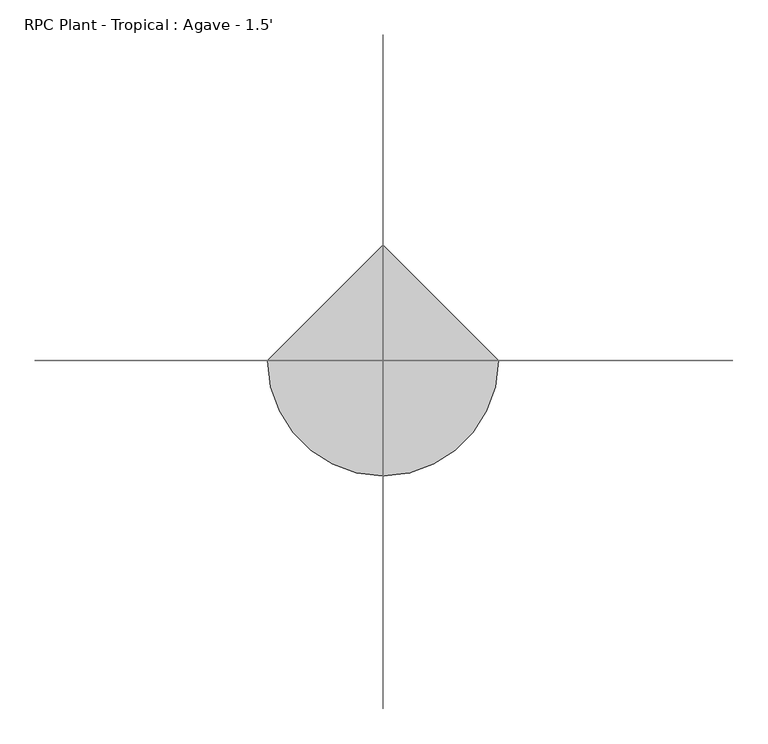
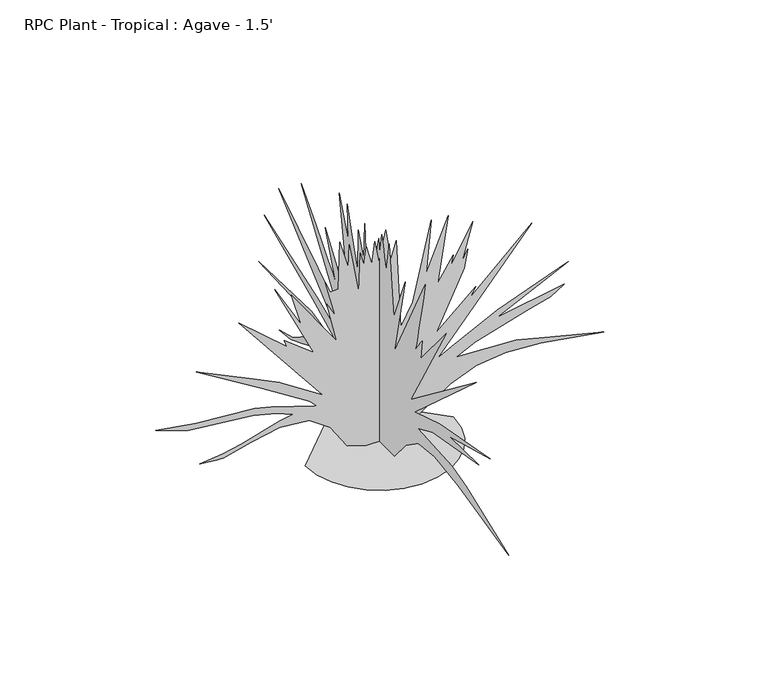
"""IFC4 building model written with IfcOpenShell, lengths in millimetres: geographic element geometry, RPC Plant - Tropical : Agave - 1.5'."""

from ifc_helpers import new_model, si_unit, origin, place, context, project, spatial, triangles, source, transform, mapped, element, save


def rpc_plant_tropical_agave_1_5_74a88192(model_context):
    return source(origin(), model_context, "Body", "Tessellation", [
        triangles([(-200.9449838, 0.0, 1.26e-05), (-195.6326446, -46.0431244, 1.26e-05), (-180.5030448, -88.3267035, 1.26e-05), (-156.767902, -125.6386611, 1.26e-05), (-125.6386611, -156.767902, 1.26e-05), (-88.3267035, -180.5030448, 1.26e-05), (-46.0431244, -195.6326446, 1.26e-05), (8.8e-06, -200.9449838, 1.26e-05), (46.0431244, -195.6326446, 1.26e-05), (88.3267035, -180.5030448, 1.26e-05), (125.6386611, -156.767902, 1.26e-05), (156.767902, -125.6386611, 1.26e-05), (180.5030448, -88.3267035, 1.26e-05), (195.6326446, -46.0431244, 1.26e-05), (200.9449838, 1.76e-05, 1.26e-05), (-2.64e-05, 200.9449838, 1.26e-05), (-33.2531301, 1.5e-06, 3.4e-06), (-87.23451, 2.8e-06, 17.5224236), (-132.8827502, 6e-07, 86.7952563), (-190.7246956, 7e-07, 127.5544962), (-269.7661646, 3.8e-06, 134.8537872), (-346.3140358, 8.1e-06, 118.9056237), (-422.3684778, 1.25e-05, 99.9853214), (-439.494867, 1.32e-05, 100.6714532), (-487.1046427, 1.5e-05, 105.5966886), (-424.417408, 1.19e-05, 112.1471881), (-376.4520218, 9.2e-06, 122.3864432), (-270.8011305, 2.7e-06, 153.1431596), (-234.2809759, 7e-07, 159.7728966), (-277.816618, 1.6e-06, 177.4516504), (-342.3583906, 3.4e-06, 194.3836474), (-519.0443356, 1e-05, 213.4357003), (-606.9487083, 1.2e-05, 243.4998354), (-498.5956201, 8.4e-06, 225.4410903), (-337.7084928, 2.1e-06, 212.3075897), (-293.8098278, 8e-07, 201.4407929), (-170.2543063, -2.2e-06, 161.4147659), (-187.2980515, -2.6e-06, 180.4058487), (-317.7989522, -1.8e-06, 262.7469528), (-496.9530968, -5e-07, 373.1940448), (-341.7894573, -2.9e-06, 298.7310027), (-272.0403172, -3.9e-06, 264.8422827), (-153.8374304, -4.5e-06, 187.6821124), (-382.0332218, -1.15e-05, 473.3378594), (-250.6978699, -1.05e-05, 360.0605441), (-257.2649473, -1.14e-05, 379.7607951), (-178.4629077, -1.11e-05, 317.3766306), (-283.5322938, -1.95e-05, 535.7236954), (-211.2970046, -1.52e-05, 409.312843), (-239.2062203, -1.96e-05, 504.532467), (-116.0780891, -1.45e-05, 328.8686254), (-142.3454357, -2.02e-05, 443.7891543), (-119.3614643, -1.88e-05, 402.7460927), (-147.270671, -2.38e-05, 507.8141344), (-132.9569099, -2.26e-05, 475.9049266), (-111.0309408, -2.35e-05, 475.9320325), (-107.8694877, -3.16e-05, 609.6005087), (-84.5692021, -2.79e-05, 529.295781), (-81.6021412, -3.18e-05, 593.1819251), (-55.3351308, -2.42e-05, 447.0708218), (-52.051415, -3.1e-05, 558.708993), (-42.2012849, -2.92e-05, 520.9476351), (-35.6345346, -3.25e-05, 571.8424936), (-20.8591737, -2.98e-05, 516.023408), (-12.6506665, -3.39e-05, 578.4092803), (-1.1586981, -3.07e-05, 516.023408), (16.9000563, -3.66e-05, 601.3911987), (31.6754171, -3.18e-05, 511.0992173), (46.4508802, -3.54e-05, 560.3481371), (57.9428658, -2.09e-05, 307.5265051), (90.7766266, -2.59e-05, 368.2698177), (140.6642974, -4.11e-05, 586.605001), (126.8944347, -3.17e-05, 438.8615481), (187.3105871, -4.29e-05, 582.6053541), (158.0866805, -3.07e-05, 399.4610461), (200.7712481, -3.65e-05, 465.1319286), (194.2044977, -3.45e-05, 435.5798807), (253.3059411, -4.34e-05, 542.2904457), (223.7552194, -3.58e-05, 437.222404), (240.1720953, -3.84e-05, 468.4136324), (231.2908968, -3.5e-05, 417.3460373), (154.8033053, -2.22e-05, 258.2751872), (261.5145425, -3.25e-05, 353.4937938), (245.0973215, -3.01e-05, 325.5852502), (414.1930684, -4.68e-05, 481.5471331), (158.0866805, -1.79e-05, 184.3983921), (211.2997297, -2.18e-05, 210.7700382), (320.6156407, -2.98e-05, 264.8422827), (512.6943234, -4.25e-05, 337.0772449), (318.9741348, -2.85e-05, 243.4998354), (502.3819078, -3.84e-05, 275.1540261), (465.5654414, -3.54e-05, 253.17588), (400.5481527, -3.15e-05, 234.7595259), (260.6113273, -2.3e-05, 194.7771735), (208.9798495, -1.92e-05, 169.6230221), (371.5074835, -2.59e-05, 161.4147659), (448.5270919, -2.8e-05, 141.4672734), (609.5564707, -3.26e-05, 100.6714532), (438.7667138, -2.68e-05, 128.2728117), (343.242312, -2.3e-05, 134.8036631), (263.2766261, -1.9e-05, 125.4744088), (193.0049343, -1.43e-05, 97.8246248), (115.3421693, -7.8e-06, 45.5100628), (44.0785186, -1.9e-06, 0.0), (1.2e-06, 26.7781575, 1.21e-05), (2.8e-06, 63.7333918, 1.32e-05), (4.9e-06, 91.2118108, 26.7772105), (8.3e-06, 132.92677, 78.8260843), (1.11e-05, 176.9572038, 107.6236088), (1.38e-05, 232.3665034, 113.1289777), (1.53e-05, 278.1119306, 97.1591404), (1.8e-05, 362.9899801, 61.1154965), (1.98e-05, 415.9778432, 40.3792577), (2.21e-05, 471.1026398, 33.361606), (1.97e-05, 407.172494, 51.8140112), (1.79e-05, 333.0020576, 99.7668755), (1.58e-05, 266.4753407, 130.2140541), (1.34e-05, 214.9972874, 128.5806599), (1.56e-05, 251.3697766, 147.1551893), (2.01e-05, 341.4880222, 162.6979724), (3.05e-05, 567.6227294, 172.7346963), (1.96e-05, 318.4244591, 179.4734928), (1.45e-05, 219.9269284, 158.3250926), (1.09e-05, 159.1792192, 128.5806599), (1.46e-05, 213.2609472, 170.2228038), (2.05e-05, 311.7594953, 220.3624396), (3.38e-05, 541.6977493, 320.6603691), (2e-05, 290.5156066, 236.9330851), (1.47e-05, 196.9382153, 197.5322379), (3.42e-05, 472.7451631, 438.8615481), (1.66e-05, 194.9377015, 264.7396727), (3.18e-05, 366.0345981, 517.6659677), (2.91e-05, 331.7090406, 479.3288455), (2.65e-05, 298.6551353, 442.1771161), (2.41e-05, 268.1432804, 407.3994061), (2.2e-05, 241.444474, 376.1810718), (2.02e-05, 219.8300593, 349.7040905), (1.9e-05, 204.5710888, 329.1615581), (1.82e-05, 196.9382153, 315.7351247), (2.51e-05, 254.3981346, 460.2043588), (2.02e-05, 198.5512891, 378.3282154), (1.97e-05, 193.2335359, 371.1213879), (1.92e-05, 186.8002077, 363.6537841), (1.86e-05, 179.4369216, 355.9694421), (1.8e-05, 171.3295677, 348.1157427), (1.74e-05, 162.6641082, 340.1299656), (1.68e-05, 153.6267783, 332.0585469), (1.61e-05, 144.4038584, 323.9437443), (2.62e-05, 187.0880898, 599.7486754), (2.11e-05, 146.0453733, 489.7564067), (2.43e-05, 150.9706087, 589.9002213), (2.15e-05, 131.2703486, 524.232718), (1.72e-05, 100.0777758, 427.3705708), (2.07e-05, 98.4359156, 547.2146364), (1.76e-05, 73.8104293, 478.2654656), (2.05e-05, 68.8851939, 583.333471), (1.81e-05, 63.0127099, 512.2439149), (1.46e-05, 36.0510948, 437.222404), (1.74e-05, 1.5752787, 581.6909477), (1.6e-05, -1.7081751, 540.6478861), (1.74e-05, -11.4000706, 600.60887), (1.66e-05, -15.9711602, 581.5250058), (1.59e-05, -20.3254695, 563.0236279), (1.52e-05, -24.246283, 545.6838796), (1.46e-05, -27.5167911, 530.0916627), (1.41e-05, -29.9202417, 516.8260843), (1.37e-05, -31.2398582, 506.4696307), (1.35e-05, -31.258891, 499.6048608), (1.57e-05, -46.0343177, 594.8244484), (8.8e-06, -67.3764334, 397.821902), (1.04e-05, -123.1944971, 532.4419916), (5.8e-06, -70.6598086, 300.9597548), (7.6e-06, -216.7715614, 581.6909477), (6.8e-06, -207.9360723, 538.6666843), (5.9e-06, -199.3546012, 497.2104939), (5.1e-06, -191.2818018, 458.8869246), (4.4e-06, -183.9716739, 425.264086), (3.9e-06, -177.6789076, 397.9099417), (3.6e-06, -172.6578296, 378.3891855), (3.4e-06, -169.1620946, 368.2698177), (3.4e-06, -168.0119831, 365.6180537), (3.4e-06, -169.5576736, 367.0032163), (3.3e-06, -173.3493753, 371.7547068), (3.3e-06, -178.9387326, 379.1985838), (3.3e-06, -185.8756638, 388.6609423), (3.2e-06, -193.7113955, 399.4711836), (3.2e-06, -201.9962096, 410.9554027), (1.9e-06, -193.7879352, 355.1363171), (8e-07, -315.274179, 501.2473841), (-3e-07, -147.8199925, 210.6657386), (-7.1e-06, -454.8195494, 445.4282985), (-1.9e-06, -165.8787194, 184.3987372), (-6.1e-06, -284.0816244, 222.1577152), (-1.54e-05, -521.71979, 265.9195789), (-8.3e-06, -328.407716, 213.9491138), (-1.45e-05, -468.6201968, 217.2328341), (-6e-06, -252.4355546, 178.0016531), (-3.7e-06, -180.6540894, 146.639396), (-1.13e-05, -343.1847573, 136.7889344), (-1.47e-05, -408.8522607, 118.7301893), (-2.59e-05, -607.4973667, 41.5700099), (-1.37e-05, -370.6743585, 97.1591404), (-8.3e-06, -260.1791771, 113.3443716), (-5.1e-06, -183.4795891, 105.2979877), (-3.7e-06, -125.5777001, 65.1557931), (-3.1e-06, -70.1362304, 9.2e-06), (-1.1e-06, -25.5007055, 1.06e-05)], [[15, 16, 1], [14, 15, 1], [14, 1, 2], [13, 14, 2], [13, 2, 3], [13, 3, 4], [12, 13, 4], [11, 12, 4], [11, 4, 5], [11, 5, 6], [11, 6, 7], [11, 7, 8], [11, 8, 9], [11, 9, 10], [47, 48, 49], [97, 98, 99], [88, 89, 90], [39, 40, 41], [84, 85, 86], [71, 72, 73], [53, 54, 55], [32, 33, 34], [43, 44, 45], [24, 25, 26], [58, 59, 60], [77, 78, 79], [73, 74, 75], [60, 61, 62], [51, 52, 53], [56, 57, 58], [82, 83, 84], [79, 80, 81], [64, 65, 66], [49, 50, 51], [68, 69, 70], [75, 76, 77], [90, 91, 92], [90, 92, 93], [66, 67, 68], [82, 84, 86], [90, 93, 94], [62, 63, 64], [47, 49, 51], [39, 41, 42], [45, 46, 47], [43, 45, 47], [38, 39, 42], [38, 42, 43], [31, 32, 34], [31, 34, 35], [23, 24, 26], [56, 58, 60], [87, 88, 90], [87, 90, 94], [87, 94, 95], [37, 38, 43], [86, 87, 95], [71, 73, 75], [96, 97, 99], [96, 99, 100], [95, 96, 100], [95, 100, 101], [95, 101, 102], [53, 55, 56], [53, 56, 60], [22, 23, 26], [22, 26, 27], [22, 27, 28], [21, 22, 28], [60, 62, 64], [43, 47, 51], [30, 31, 35], [30, 35, 36], [30, 36, 37], [29, 30, 37], [86, 95, 102], [21, 28, 29], [20, 21, 29], [20, 29, 37], [19, 20, 37], [86, 102, 103], [66, 68, 70], [64, 66, 70], [60, 64, 70], [53, 60, 70], [51, 53, 70], [43, 51, 70], [77, 79, 81], [77, 81, 82], [75, 77, 82], [71, 75, 82], [70, 71, 82], [70, 82, 86], [43, 70, 86], [43, 86, 103], [43, 103, 104], [43, 104, 17], [43, 17, 18], [43, 18, 19], [43, 19, 37], [120, 121, 122], [193, 194, 195], [190, 191, 192], [126, 127, 128], [155, 156, 157], [131, 132, 133], [200, 201, 202], [113, 114, 115], [195, 196, 197], [129, 130, 131], [131, 133, 134], [170, 171, 172], [188, 189, 190], [131, 134, 135], [148, 149, 150], [139, 140, 141], [131, 135, 136], [150, 151, 152], [168, 169, 170], [172, 173, 174], [131, 136, 137], [158, 159, 160], [172, 174, 175], [131, 137, 138], [153, 154, 155], [131, 138, 139], [172, 175, 176], [160, 161, 162], [172, 176, 177], [186, 187, 188], [172, 177, 178], [112, 113, 115], [112, 115, 116], [111, 112, 116], [111, 116, 117], [160, 162, 163], [172, 178, 179], [172, 179, 180], [172, 180, 181], [139, 141, 142], [193, 195, 197], [185, 186, 188], [192, 193, 197], [192, 197, 198], [155, 157, 158], [150, 152, 153], [148, 150, 153], [139, 142, 143], [199, 200, 202], [119, 120, 122], [119, 122, 123], [118, 119, 123], [199, 202, 203], [198, 199, 203], [198, 203, 204], [184, 185, 188], [110, 111, 117], [110, 117, 118], [109, 110, 118], [160, 163, 164], [118, 123, 124], [109, 118, 124], [139, 143, 144], [125, 126, 128], [125, 128, 129], [183, 184, 188], [139, 144, 145], [153, 155, 158], [108, 109, 124], [139, 145, 146], [160, 164, 165], [158, 160, 165], [158, 165, 166], [158, 166, 167], [158, 167, 168], [158, 168, 170], [182, 183, 188], [124, 125, 129], [182, 188, 190], [181, 182, 190], [172, 181, 190], [139, 146, 147], [131, 139, 147], [131, 147, 148], [158, 170, 172], [153, 158, 172], [148, 153, 172], [198, 204, 205], [131, 148, 172], [129, 131, 172], [124, 129, 172], [124, 172, 190], [108, 124, 190], [107, 108, 190], [106, 107, 190], [105, 106, 190], [207, 105, 190], [206, 207, 190], [205, 206, 190], [198, 205, 190], [192, 198, 190]], closed=False),
    ])


if __name__ == "__main__":
    model = new_model("IFC4")
    model_context = context("Model", 3, world=origin())
    ifc_project = project(units=[si_unit("LENGTHUNIT", "METRE", prefix="MILLI")], contexts=[model_context])
    site = spatial("IfcSite", under=ifc_project)
    building = spatial("IfcBuilding", under=site)
    placement = place(None, origin())
    rpc_plant_tropical_agave_1_5_shape = rpc_plant_tropical_agave_1_5_74a88192(model_context)
    element("IfcGeographicElement", 1, ObjectType="RPC Plant - Tropical : Agave - 1.5'", at=placement, inside=building, context=model_context, shape_type="MappedRepresentation", body=[
        mapped(rpc_plant_tropical_agave_1_5_shape, transform((0.0, 0.0, 0.0), x_axis=(1.0, 0.0, 0.0), y_axis=(0.0, 1.0, 0.0), z_axis=(0.0, 0.0, 1.0))),
    ])
    save(model, "model.ifc")

# Revit data of these elements
# Type "RPC Plant - Tropical : Agave - 1.5'"
#   built-in parameter 1005198 = "{2, 15},{39, RPC-16-G1GJ-63FX-7K5P-N000-ST1L-LVER-AU},{1, 0},{1, 0},{2, 13},{1, 8},{5, Color},{1, 0},{1, 0},{3, 0.8},{3, 0.8},{3, 0.8},{1, 8},{7, BBoxMin},{1, 0},{1, 0},{1, 0},{1, 0},{1, 0},{1, 8},{7, BBoxMax},{1, 0},{1, 0},{1, 0},{1, 0},{1, 0},{2, 11},{9, RPCTypeId},{1, 0},{1, 0},{39, RPC-16-G1GJ-63FX-7K5P-N000-ST1L-LVER-AU},{1, 6},{14, RPCPlantHeight},{1, 0},{1, 0},{3, 1.5},{2, 11},{7, keyword},{1, 0},{1, 0},{35, :RPCs:Plants [General]:Geometry:RPC},{2, 11},{8, category},{1, 0},{1, 0},{16, Plants [General]},{2, 11},{12, LocalizedUID},{1, 0},{1, 0},{5, Agave},{2, 14},{6, Height},{1, 0},{1, 0},{3, 1.5},{1, 2},{16, Cast Reflections},{1, 0},{1, 0},{1, 0},{1, 2},{12, Cast Shadows},{1, 0},{1, 0},{1, 1},{1, 2},{9, Lock View},{1, 0},{1, 0},{1, 0},{1, 4},{5, ViewC},{1, 0},{1, 0},{1, 0},{21, assetlibrary_base.fbx},{1, 5},"
#   built-in parameter 1005195 = "RPC-16-G1GJ-63FX-7K5P-N000-ST1L-LVER-AU"
#   Type Comments = "Agave"
#   Assembly Code = "G2050500"
#   Height = 2' - 0"
#   Default Elevation = 0
